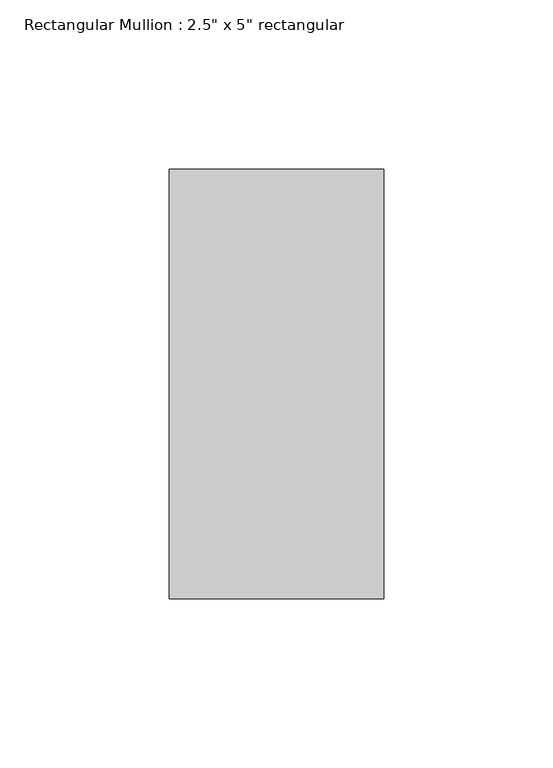
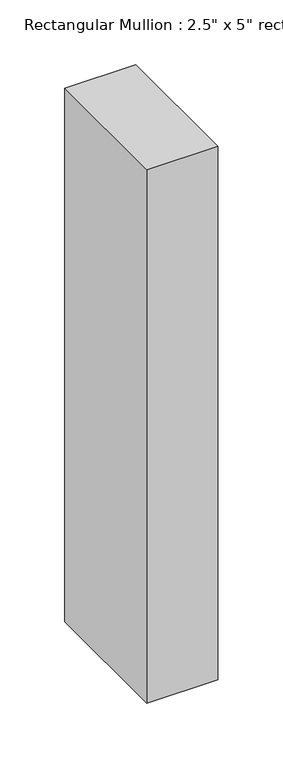
"""IFC4 building model written with IfcOpenShell, lengths in millimetres: member geometry."""

from ifc_helpers import new_model, si_unit, frame, origin, place, context, project, spatial, polyline, outline, extrude, source, transform, mapped, element, save


def member_67dd967c(model_context):
    return source(origin(), model_context, "Body", "SweptSolid", [
        extrude(outline(polyline([(0.0, 63.5), (0.0, -63.5), (-63.5, -63.5), (-63.5, 63.5), (0.0, 63.5)])), frame((0.0, 0.0, -503.7666667), z_axis=(0.0, 0.0, 1.0), x_axis=(1.0, 0.0, 0.0)), (0.0, 0.0, 1.0), 503.7666667),
    ])


if __name__ == "__main__":
    model = new_model("IFC4")
    model_context = context("Model", 3, world=origin())
    ifc_project = project(units=[si_unit("LENGTHUNIT", "METRE", prefix="MILLI")], contexts=[model_context])
    site = spatial("IfcSite", under=ifc_project)
    building = spatial("IfcBuilding", under=site)
    placement = place(None, origin())
    member_shape = member_67dd967c(model_context)
    element("IfcMember", 1, ObjectType="Rectangular Mullion : 2.5\" x 5\" rectangular", at=placement, inside=building, context=model_context, shape_type="MappedRepresentation", body=[
        mapped(member_shape, transform((0.0, 0.0, 0.0), x_axis=(1.0, 0.0, 0.0), y_axis=(0.0, 1.0, 0.0), z_axis=(0.0, 0.0, 1.0))),
    ])
    save(model, "model.ifc")

# Revit data of these elements
# Type "Rectangular Mullion : 2.5\" x 5\" rectangular"
#   built-in parameter 1007304 = 0.416667 (stored number, unit not read)
#   built-in parameter 1007301 = 0.104167 (stored number, unit not read)
#   built-in parameter 1007300 = 0.104167 (stored number, unit not read)
# Element 1 (IfcMember, "Rectangular Mullion : 2.5\" x 5\" rectangular")
#   Materials on its faces: "Aluminum"
# Materials
#   "Aluminum": class "Metal", colour RGB 247 247 247, transparency 0, Description = "Aluminum 6061", Cost = 0
